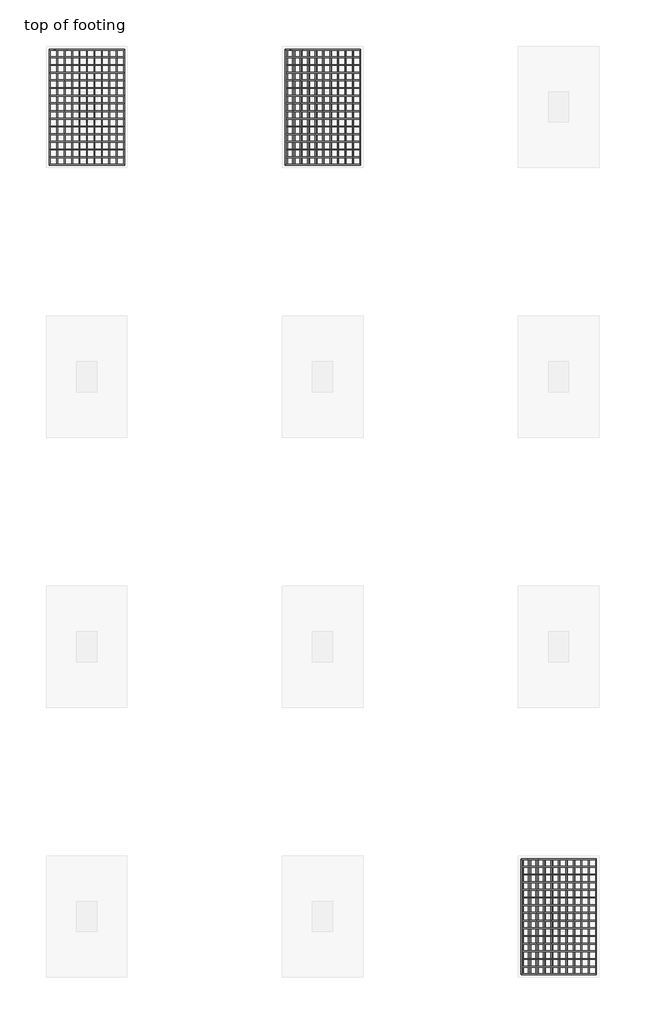
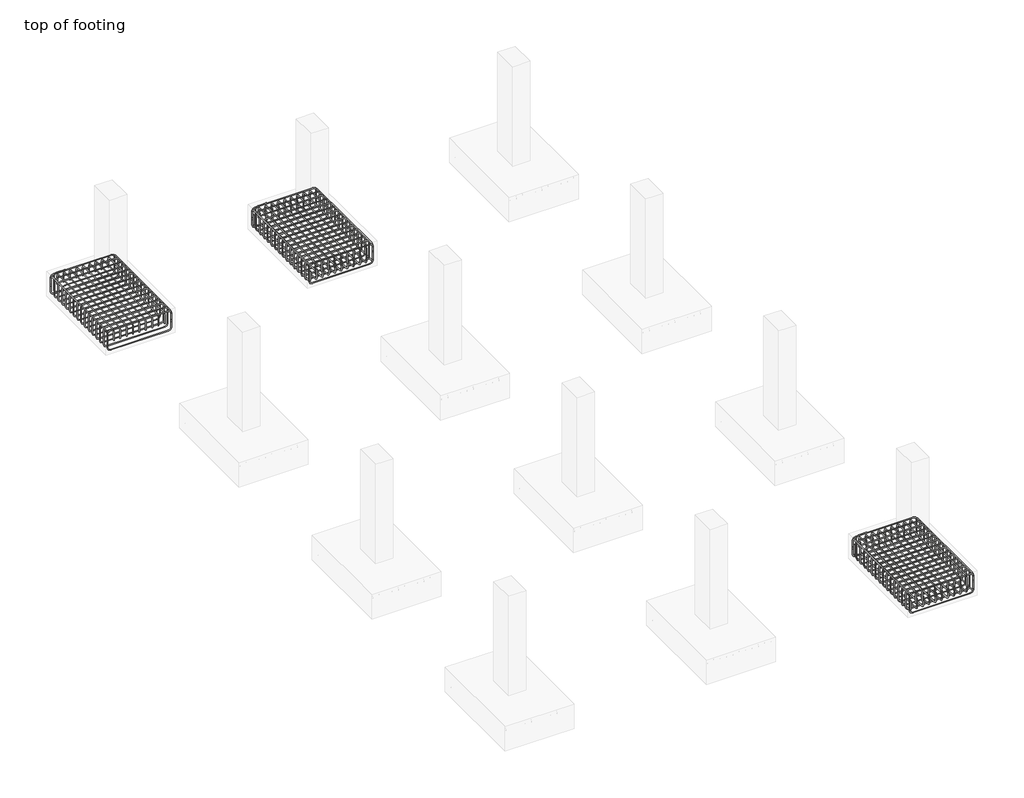
# One storey, part 7 of 8: 14 reinforcing bars.
"""IFC4 building model written with IfcOpenShell, lengths in millimetres."""

from ifc_helpers import new_model, si_unit, point, frame, origin, place, context, project, spatial, polyline, circle_curve, trimmed, segment, composite_curve, source, transform, mapped, element, save
from ifc_brep_helpers import swept_disk

model = new_model("IFC4")

# Units and contexts
model_context = context("Model", 3, world=origin())
ifc_project = project(units=[si_unit("LENGTHUNIT", "METRE", prefix="MILLI")], contexts=[model_context])

# Site, building, storey
site = spatial("IfcSite", under=ifc_project)
building = spatial("IfcBuilding", under=site)
storey = spatial("IfcBuildingStorey", under=building, Name="top of footing", Elevation=-1828.8)

# Reinforcing bars
placement = place(None, origin())
reinforcing_bar_shape = source(origin(), model_context, "Body", "SolidModel", [
    swept_disk(composite_curve([segment(polyline([(3314.5699811, 4682.8075251, -2014.4920065), (3314.5699811, 4682.8075251, -2161.7920065)]), True, "CONTINUOUS"), segment(trimmed(circle_curve(frame((3314.5699811, 4729.1575251, -2161.7920065), z_axis=(1.0, 0.0, 0.0), x_axis=(0.0, -46.350000000000364, 0.0)), 46.35), [point((3314.5699811, 4682.8075251, -2161.7920065))], [point((3314.5699811, 4729.1575251, -2208.1420065))], True, "CARTESIAN"), True, "CONTINUOUS"), segment(polyline([(3314.5699811, 4729.1575251, -2208.1420065), (3314.5699811, 6343.7575251, -2208.1420065)]), True, "CONTINUOUS"), segment(trimmed(circle_curve(frame((3314.5699811, 6343.7575251, -2161.7920065), z_axis=(1.0, 0.0, 0.0), x_axis=(0.0, 0.0, -46.350000000000364)), 46.35), [point((3314.5699811, 6343.7575251, -2208.1420065))], [point((3314.5699811, 6390.1075251, -2161.7920065))], True, "CARTESIAN"), True, "CONTINUOUS"), segment(polyline([(3314.5699811, 6390.1075251, -2161.7920065), (3314.5699811, 6390.1075251, -2014.4920065)]), True, "CONTINUOUS")], self_intersect=False), 6.35),
])
element("IfcReinforcingBar", 1, at=placement, inside=storey, context=model_context, shape_type="MappedRepresentation", body=[
    mapped(reinforcing_bar_shape, transform((0.0, 0.0, 0.0), x_axis=(1.0, 0.0, 0.0), y_axis=(0.0, 1.0, 0.0), z_axis=(0.0, 0.0, 1.0))),
    mapped(reinforcing_bar_shape, transform((-108.3645139, 0.0, 0.0), x_axis=(1.0, 0.0, 0.0), y_axis=(0.0, 1.0, 0.0), z_axis=(0.0, 0.0, 1.0))),
    mapped(reinforcing_bar_shape, transform((-216.7290279, 0.0, 0.0), x_axis=(1.0, 0.0, 0.0), y_axis=(0.0, 1.0, 0.0), z_axis=(0.0, 0.0, 1.0))),
    mapped(reinforcing_bar_shape, transform((-325.0935418, 0.0, 0.0), x_axis=(1.0, 0.0, 0.0), y_axis=(0.0, 1.0, 0.0), z_axis=(0.0, 0.0, 1.0))),
    mapped(reinforcing_bar_shape, transform((-433.4580557, 0.0, 0.0), x_axis=(1.0, 0.0, 0.0), y_axis=(0.0, 1.0, 0.0), z_axis=(0.0, 0.0, 1.0))),
    mapped(reinforcing_bar_shape, transform((-541.8225696, 0.0, 0.0), x_axis=(1.0, 0.0, 0.0), y_axis=(0.0, 1.0, 0.0), z_axis=(0.0, 0.0, 1.0))),
    mapped(reinforcing_bar_shape, transform((-650.1870836, 0.0, 0.0), x_axis=(1.0, 0.0, 0.0), y_axis=(0.0, 1.0, 0.0), z_axis=(0.0, 0.0, 1.0))),
    mapped(reinforcing_bar_shape, transform((-758.5515975, 0.0, 0.0), x_axis=(1.0, 0.0, 0.0), y_axis=(0.0, 1.0, 0.0), z_axis=(0.0, 0.0, 1.0))),
    mapped(reinforcing_bar_shape, transform((-866.9161114, 0.0, 0.0), x_axis=(1.0, 0.0, 0.0), y_axis=(0.0, 1.0, 0.0), z_axis=(0.0, 0.0, 1.0))),
    mapped(reinforcing_bar_shape, transform((-975.2806253, 0.0, 0.0), x_axis=(1.0, 0.0, 0.0), y_axis=(0.0, 1.0, 0.0), z_axis=(0.0, 0.0, 1.0))),
    mapped(reinforcing_bar_shape, transform((-1083.6451393, 0.0, 0.0), x_axis=(1.0, 0.0, 0.0), y_axis=(0.0, 1.0, 0.0), z_axis=(0.0, 0.0, 1.0))),
])
reinforcing_bar_2_shape = source(origin(), model_context, "Body", "SolidModel", [
    swept_disk(composite_curve([segment(polyline([(2207.2699811, 4682.8075251, -2085.8010212), (2207.2699811, 4682.8075251, -1938.5010212)]), True, "CONTINUOUS"), segment(trimmed(circle_curve(frame((2207.2699811, 4729.1575251, -1938.5010212), z_axis=(-1.0, 0.0, 0.0), x_axis=(0.0, -46.350000000000364, 0.0)), 46.35), [point((2207.2699811, 4682.8075251, -1938.5010212))], [point((2207.2699811, 4729.1575251, -1892.1510212))], True, "CARTESIAN"), True, "CONTINUOUS"), segment(polyline([(2207.2699811, 4729.1575251, -1892.1510212), (2207.2699811, 6343.7575251, -1892.1510212)]), True, "CONTINUOUS"), segment(trimmed(circle_curve(frame((2207.2699811, 6343.7575251, -1938.5010212), z_axis=(-1.0, 0.0, 0.0), x_axis=(0.0, 0.0, 46.34999999999991)), 46.35), [point((2207.2699811, 6343.7575251, -1892.1510212))], [point((2207.2699811, 6390.1075251, -1938.5010212))], True, "CARTESIAN"), True, "CONTINUOUS"), segment(polyline([(2207.2699811, 6390.1075251, -1938.5010212), (2207.2699811, 6390.1075251, -2085.8010212)]), True, "CONTINUOUS")], self_intersect=False), 6.35),
])
element("IfcReinforcingBar", 2, at=placement, inside=storey, context=model_context, shape_type="MappedRepresentation", body=[
    mapped(reinforcing_bar_2_shape, transform((0.0, 0.0, 0.0), x_axis=(1.0, 0.0, 0.0), y_axis=(0.0, 1.0, 0.0), z_axis=(0.0, 0.0, 1.0))),
    mapped(reinforcing_bar_2_shape, transform((110.73, 0.0, 0.0), x_axis=(1.0, 0.0, 0.0), y_axis=(0.0, 1.0, 0.0), z_axis=(0.0, 0.0, 1.0))),
    mapped(reinforcing_bar_2_shape, transform((221.46, 0.0, 0.0), x_axis=(1.0, 0.0, 0.0), y_axis=(0.0, 1.0, 0.0), z_axis=(0.0, 0.0, 1.0))),
    mapped(reinforcing_bar_2_shape, transform((332.19, 0.0, 0.0), x_axis=(1.0, 0.0, 0.0), y_axis=(0.0, 1.0, 0.0), z_axis=(0.0, 0.0, 1.0))),
    mapped(reinforcing_bar_2_shape, transform((442.92, 0.0, 0.0), x_axis=(1.0, 0.0, 0.0), y_axis=(0.0, 1.0, 0.0), z_axis=(0.0, 0.0, 1.0))),
    mapped(reinforcing_bar_2_shape, transform((553.65, 0.0, 0.0), x_axis=(1.0, 0.0, 0.0), y_axis=(0.0, 1.0, 0.0), z_axis=(0.0, 0.0, 1.0))),
    mapped(reinforcing_bar_2_shape, transform((664.38, 0.0, 0.0), x_axis=(1.0, 0.0, 0.0), y_axis=(0.0, 1.0, 0.0), z_axis=(0.0, 0.0, 1.0))),
    mapped(reinforcing_bar_2_shape, transform((775.11, 0.0, 0.0), x_axis=(1.0, 0.0, 0.0), y_axis=(0.0, 1.0, 0.0), z_axis=(0.0, 0.0, 1.0))),
    mapped(reinforcing_bar_2_shape, transform((885.84, 0.0, 0.0), x_axis=(1.0, 0.0, 0.0), y_axis=(0.0, 1.0, 0.0), z_axis=(0.0, 0.0, 1.0))),
    mapped(reinforcing_bar_2_shape, transform((996.57, 0.0, 0.0), x_axis=(1.0, 0.0, 0.0), y_axis=(0.0, 1.0, 0.0), z_axis=(0.0, 0.0, 1.0))),
    mapped(reinforcing_bar_2_shape, transform((1107.3, 0.0, 0.0), x_axis=(1.0, 0.0, 0.0), y_axis=(0.0, 1.0, 0.0), z_axis=(0.0, 0.0, 1.0))),
])
element("IfcReinforcingBar", 3, at=placement, inside=storey, context=model_context, shape_type="SolidModel", body=[
    swept_disk(composite_curve([segment(polyline([(2456.9690895, 6390.1075251, -2232.45), (2309.6690895, 6390.1075251, -2232.45)]), True, "CONTINUOUS"), segment(trimmed(circle_curve(frame((2309.6690895, 6390.1075251, -2186.1), z_axis=(0.0, 1.0, 0.0), x_axis=(0.0, 0.0, -46.34999999999991)), 46.35), [point((2309.6690895, 6390.1075251, -2232.45))], [point((2263.3190895, 6390.1075251, -2186.1))], True, "CARTESIAN"), True, "CONTINUOUS"), segment(polyline([(2263.3190895, 6390.1075251, -2186.1), (2263.3190895, 6390.1075251, -1921.5)]), True, "CONTINUOUS"), segment(trimmed(circle_curve(frame((2309.6690895, 6390.1075251, -1921.5), z_axis=(0.0, 1.0, 0.0), x_axis=(-46.350000000000364, 0.0, 0.0)), 46.35), [point((2263.3190895, 6390.1075251, -1921.5))], [point((2309.6690895, 6390.1075251, -1875.15))], True, "CARTESIAN"), True, "CONTINUOUS"), segment(polyline([(2309.6690895, 6390.1075251, -1875.15), (2456.9690895, 6390.1075251, -1875.15)]), True, "CONTINUOUS")], self_intersect=False), 6.35),
])
reinforcing_bar_3_shape = source(origin(), model_context, "Body", "SolidModel", [
    swept_disk(composite_curve([segment(polyline([(3314.5699811, 6390.1075251, -2044.8290141), (3314.5699811, 6390.1075251, -2192.1290141)]), True, "CONTINUOUS"), segment(trimmed(circle_curve(frame((3268.2199811, 6390.1075251, -2192.1290141), z_axis=(0.0, 1.0, 0.0), x_axis=(46.34999999999991, 0.0, 0.0)), 46.35), [point((3314.5699811, 6390.1075251, -2192.1290141))], [point((3268.2199811, 6390.1075251, -2238.4790141))], True, "CARTESIAN"), True, "CONTINUOUS"), segment(polyline([(3268.2199811, 6390.1075251, -2238.4790141), (2253.6199811, 6390.1075251, -2238.4790141)]), True, "CONTINUOUS"), segment(trimmed(circle_curve(frame((2253.6199811, 6390.1075251, -2192.1290141), z_axis=(0.0, 1.0, 0.0), x_axis=(0.0, 0.0, -46.34999999999991)), 46.35), [point((2253.6199811, 6390.1075251, -2238.4790141))], [point((2207.2699811, 6390.1075251, -2192.1290141))], True, "CARTESIAN"), True, "CONTINUOUS"), segment(polyline([(2207.2699811, 6390.1075251, -2192.1290141), (2207.2699811, 6390.1075251, -2044.8290141)]), True, "CONTINUOUS")], self_intersect=False), 6.35),
])
element("IfcReinforcingBar", 4, at=placement, inside=storey, context=model_context, shape_type="MappedRepresentation", body=[
    mapped(reinforcing_bar_3_shape, transform((0.0, 0.0, 0.0), x_axis=(1.0, 0.0, 0.0), y_axis=(0.0, 1.0, 0.0), z_axis=(0.0, 0.0, 1.0))),
    mapped(reinforcing_bar_3_shape, transform((0.0, -113.82, 0.0), x_axis=(1.0, 0.0, 0.0), y_axis=(0.0, 1.0, 0.0), z_axis=(0.0, 0.0, 1.0))),
    mapped(reinforcing_bar_3_shape, transform((0.0, -227.64, 0.0), x_axis=(1.0, 0.0, 0.0), y_axis=(0.0, 1.0, 0.0), z_axis=(0.0, 0.0, 1.0))),
    mapped(reinforcing_bar_3_shape, transform((0.0, -341.46, 0.0), x_axis=(1.0, 0.0, 0.0), y_axis=(0.0, 1.0, 0.0), z_axis=(0.0, 0.0, 1.0))),
    mapped(reinforcing_bar_3_shape, transform((0.0, -455.28, 0.0), x_axis=(1.0, 0.0, 0.0), y_axis=(0.0, 1.0, 0.0), z_axis=(0.0, 0.0, 1.0))),
    mapped(reinforcing_bar_3_shape, transform((0.0, -569.1, 0.0), x_axis=(1.0, 0.0, 0.0), y_axis=(0.0, 1.0, 0.0), z_axis=(0.0, 0.0, 1.0))),
    mapped(reinforcing_bar_3_shape, transform((0.0, -682.92, 0.0), x_axis=(1.0, 0.0, 0.0), y_axis=(0.0, 1.0, 0.0), z_axis=(0.0, 0.0, 1.0))),
    mapped(reinforcing_bar_3_shape, transform((0.0, -796.74, 0.0), x_axis=(1.0, 0.0, 0.0), y_axis=(0.0, 1.0, 0.0), z_axis=(0.0, 0.0, 1.0))),
    mapped(reinforcing_bar_3_shape, transform((0.0, -910.56, 0.0), x_axis=(1.0, 0.0, 0.0), y_axis=(0.0, 1.0, 0.0), z_axis=(0.0, 0.0, 1.0))),
    mapped(reinforcing_bar_3_shape, transform((0.0, -1024.38, 0.0), x_axis=(1.0, 0.0, 0.0), y_axis=(0.0, 1.0, 0.0), z_axis=(0.0, 0.0, 1.0))),
    mapped(reinforcing_bar_3_shape, transform((0.0, -1138.2, 0.0), x_axis=(1.0, 0.0, 0.0), y_axis=(0.0, 1.0, 0.0), z_axis=(0.0, 0.0, 1.0))),
    mapped(reinforcing_bar_3_shape, transform((0.0, -1252.02, 0.0), x_axis=(1.0, 0.0, 0.0), y_axis=(0.0, 1.0, 0.0), z_axis=(0.0, 0.0, 1.0))),
    mapped(reinforcing_bar_3_shape, transform((0.0, -1365.84, 0.0), x_axis=(1.0, 0.0, 0.0), y_axis=(0.0, 1.0, 0.0), z_axis=(0.0, 0.0, 1.0))),
    mapped(reinforcing_bar_3_shape, transform((0.0, -1479.66, 0.0), x_axis=(1.0, 0.0, 0.0), y_axis=(0.0, 1.0, 0.0), z_axis=(0.0, 0.0, 1.0))),
    mapped(reinforcing_bar_3_shape, transform((0.0, -1593.48, 0.0), x_axis=(1.0, 0.0, 0.0), y_axis=(0.0, 1.0, 0.0), z_axis=(0.0, 0.0, 1.0))),
    mapped(reinforcing_bar_3_shape, transform((0.0, -1707.3, 0.0), x_axis=(1.0, 0.0, 0.0), y_axis=(0.0, 1.0, 0.0), z_axis=(0.0, 0.0, 1.0))),
])
reinforcing_bar_4_shape = source(origin(), model_context, "Body", "SolidModel", [
    swept_disk(composite_curve([segment(polyline([(2207.2699811, 6390.1075251, -2075.0801535), (2207.2699811, 6390.1075251, -1927.7801535)]), True, "CONTINUOUS"), segment(trimmed(circle_curve(frame((2253.6199811, 6390.1075251, -1927.7801535), z_axis=(0.0, 1.0, 0.0), x_axis=(-46.34999999999991, 0.0, 0.0)), 46.35), [point((2207.2699811, 6390.1075251, -1927.7801535))], [point((2253.6199811, 6390.1075251, -1881.4301535))], True, "CARTESIAN"), True, "CONTINUOUS"), segment(polyline([(2253.6199811, 6390.1075251, -1881.4301535), (3268.2199811, 6390.1075251, -1881.4301535)]), True, "CONTINUOUS"), segment(trimmed(circle_curve(frame((3268.2199811, 6390.1075251, -1927.7801535), z_axis=(0.0, 1.0, 0.0), x_axis=(0.0, 0.0, 46.350000000000136)), 46.35), [point((3268.2199811, 6390.1075251, -1881.4301535))], [point((3314.5699811, 6390.1075251, -1927.7801535))], True, "CARTESIAN"), True, "CONTINUOUS"), segment(polyline([(3314.5699811, 6390.1075251, -1927.7801535), (3314.5699811, 6390.1075251, -2075.0801535)]), True, "CONTINUOUS")], self_intersect=False), 6.35),
])
element("IfcReinforcingBar", 5, at=placement, inside=storey, context=model_context, shape_type="MappedRepresentation", body=[
    mapped(reinforcing_bar_4_shape, transform((0.0, 0.0, 0.0), x_axis=(1.0, 0.0, 0.0), y_axis=(0.0, 1.0, 0.0), z_axis=(0.0, 0.0, 1.0))),
    mapped(reinforcing_bar_4_shape, transform((0.0, -113.82, 0.0), x_axis=(1.0, 0.0, 0.0), y_axis=(0.0, 1.0, 0.0), z_axis=(0.0, 0.0, 1.0))),
    mapped(reinforcing_bar_4_shape, transform((0.0, -227.64, 0.0), x_axis=(1.0, 0.0, 0.0), y_axis=(0.0, 1.0, 0.0), z_axis=(0.0, 0.0, 1.0))),
    mapped(reinforcing_bar_4_shape, transform((0.0, -341.46, 0.0), x_axis=(1.0, 0.0, 0.0), y_axis=(0.0, 1.0, 0.0), z_axis=(0.0, 0.0, 1.0))),
    mapped(reinforcing_bar_4_shape, transform((0.0, -455.28, 0.0), x_axis=(1.0, 0.0, 0.0), y_axis=(0.0, 1.0, 0.0), z_axis=(0.0, 0.0, 1.0))),
    mapped(reinforcing_bar_4_shape, transform((0.0, -569.1, 0.0), x_axis=(1.0, 0.0, 0.0), y_axis=(0.0, 1.0, 0.0), z_axis=(0.0, 0.0, 1.0))),
    mapped(reinforcing_bar_4_shape, transform((0.0, -682.92, 0.0), x_axis=(1.0, 0.0, 0.0), y_axis=(0.0, 1.0, 0.0), z_axis=(0.0, 0.0, 1.0))),
    mapped(reinforcing_bar_4_shape, transform((0.0, -796.74, 0.0), x_axis=(1.0, 0.0, 0.0), y_axis=(0.0, 1.0, 0.0), z_axis=(0.0, 0.0, 1.0))),
    mapped(reinforcing_bar_4_shape, transform((0.0, -910.56, 0.0), x_axis=(1.0, 0.0, 0.0), y_axis=(0.0, 1.0, 0.0), z_axis=(0.0, 0.0, 1.0))),
    mapped(reinforcing_bar_4_shape, transform((0.0, -1024.38, 0.0), x_axis=(1.0, 0.0, 0.0), y_axis=(0.0, 1.0, 0.0), z_axis=(0.0, 0.0, 1.0))),
    mapped(reinforcing_bar_4_shape, transform((0.0, -1138.2, 0.0), x_axis=(1.0, 0.0, 0.0), y_axis=(0.0, 1.0, 0.0), z_axis=(0.0, 0.0, 1.0))),
    mapped(reinforcing_bar_4_shape, transform((0.0, -1252.02, 0.0), x_axis=(1.0, 0.0, 0.0), y_axis=(0.0, 1.0, 0.0), z_axis=(0.0, 0.0, 1.0))),
    mapped(reinforcing_bar_4_shape, transform((0.0, -1365.84, 0.0), x_axis=(1.0, 0.0, 0.0), y_axis=(0.0, 1.0, 0.0), z_axis=(0.0, 0.0, 1.0))),
    mapped(reinforcing_bar_4_shape, transform((0.0, -1479.66, 0.0), x_axis=(1.0, 0.0, 0.0), y_axis=(0.0, 1.0, 0.0), z_axis=(0.0, 0.0, 1.0))),
    mapped(reinforcing_bar_4_shape, transform((0.0, -1593.48, 0.0), x_axis=(1.0, 0.0, 0.0), y_axis=(0.0, 1.0, 0.0), z_axis=(0.0, 0.0, 1.0))),
    mapped(reinforcing_bar_4_shape, transform((0.0, -1707.3, 0.0), x_axis=(1.0, 0.0, 0.0), y_axis=(0.0, 1.0, 0.0), z_axis=(0.0, 0.0, 1.0))),
])
reinforcing_bar_5_shape = source(origin(), model_context, "Body", "SolidModel", [
    swept_disk(composite_curve([segment(polyline([(-4792.7300189, 16682.8075251, -2085.8010212), (-4792.7300189, 16682.8075251, -1938.5010212)]), True, "CONTINUOUS"), segment(trimmed(circle_curve(frame((-4792.7300189, 16729.1575251, -1938.5010212), z_axis=(-1.0, 0.0, 0.0), x_axis=(0.0, -46.349999999998545, 0.0)), 46.35), [point((-4792.7300189, 16682.8075251, -1938.5010212))], [point((-4792.7300189, 16729.1575251, -1892.1510212))], True, "CARTESIAN"), True, "CONTINUOUS"), segment(polyline([(-4792.7300189, 16729.1575251, -1892.1510212), (-4792.7300189, 18343.7575251, -1892.1510212)]), True, "CONTINUOUS"), segment(trimmed(circle_curve(frame((-4792.7300189, 18343.7575251, -1938.5010212), z_axis=(-1.0, 0.0, 0.0), x_axis=(0.0, 0.0, 46.34999999999991)), 46.35), [point((-4792.7300189, 18343.7575251, -1892.1510212))], [point((-4792.7300189, 18390.1075251, -1938.5010212))], True, "CARTESIAN"), True, "CONTINUOUS"), segment(polyline([(-4792.7300189, 18390.1075251, -1938.5010212), (-4792.7300189, 18390.1075251, -2085.8010212)]), True, "CONTINUOUS")], self_intersect=False), 6.35),
])
element("IfcReinforcingBar", 6, at=placement, inside=storey, context=model_context, shape_type="MappedRepresentation", body=[
    mapped(reinforcing_bar_5_shape, transform((0.0, 0.0, 0.0), x_axis=(1.0, 0.0, 0.0), y_axis=(0.0, 1.0, 0.0), z_axis=(0.0, 0.0, 1.0))),
    mapped(reinforcing_bar_5_shape, transform((110.73, 0.0, 0.0), x_axis=(1.0, 0.0, 0.0), y_axis=(0.0, 1.0, 0.0), z_axis=(0.0, 0.0, 1.0))),
    mapped(reinforcing_bar_5_shape, transform((221.46, 0.0, 0.0), x_axis=(1.0, 0.0, 0.0), y_axis=(0.0, 1.0, 0.0), z_axis=(0.0, 0.0, 1.0))),
    mapped(reinforcing_bar_5_shape, transform((332.19, 0.0, 0.0), x_axis=(1.0, 0.0, 0.0), y_axis=(0.0, 1.0, 0.0), z_axis=(0.0, 0.0, 1.0))),
    mapped(reinforcing_bar_5_shape, transform((442.92, 0.0, 0.0), x_axis=(1.0, 0.0, 0.0), y_axis=(0.0, 1.0, 0.0), z_axis=(0.0, 0.0, 1.0))),
    mapped(reinforcing_bar_5_shape, transform((553.65, 0.0, 0.0), x_axis=(1.0, 0.0, 0.0), y_axis=(0.0, 1.0, 0.0), z_axis=(0.0, 0.0, 1.0))),
    mapped(reinforcing_bar_5_shape, transform((664.38, 0.0, 0.0), x_axis=(1.0, 0.0, 0.0), y_axis=(0.0, 1.0, 0.0), z_axis=(0.0, 0.0, 1.0))),
    mapped(reinforcing_bar_5_shape, transform((775.11, 0.0, 0.0), x_axis=(1.0, 0.0, 0.0), y_axis=(0.0, 1.0, 0.0), z_axis=(0.0, 0.0, 1.0))),
    mapped(reinforcing_bar_5_shape, transform((885.84, 0.0, 0.0), x_axis=(1.0, 0.0, 0.0), y_axis=(0.0, 1.0, 0.0), z_axis=(0.0, 0.0, 1.0))),
    mapped(reinforcing_bar_5_shape, transform((996.57, 0.0, 0.0), x_axis=(1.0, 0.0, 0.0), y_axis=(0.0, 1.0, 0.0), z_axis=(0.0, 0.0, 1.0))),
    mapped(reinforcing_bar_5_shape, transform((1107.3, 0.0, 0.0), x_axis=(1.0, 0.0, 0.0), y_axis=(0.0, 1.0, 0.0), z_axis=(0.0, 0.0, 1.0))),
])
element("IfcReinforcingBar", 7, at=placement, inside=storey, context=model_context, shape_type="SolidModel", body=[
    swept_disk(composite_curve([segment(polyline([(-4543.0309105, 18390.1075251, -2232.45), (-4690.3309105, 18390.1075251, -2232.45)]), True, "CONTINUOUS"), segment(trimmed(circle_curve(frame((-4690.3309105, 18390.1075251, -2186.1), z_axis=(0.0, 1.0, 0.0), x_axis=(0.0, 0.0, -46.34999999999991)), 46.35), [point((-4690.3309105, 18390.1075251, -2232.45))], [point((-4736.6809105, 18390.1075251, -2186.1))], True, "CARTESIAN"), True, "CONTINUOUS"), segment(polyline([(-4736.6809105, 18390.1075251, -2186.1), (-4736.6809105, 18390.1075251, -1921.5)]), True, "CONTINUOUS"), segment(trimmed(circle_curve(frame((-4690.3309105, 18390.1075251, -1921.5), z_axis=(0.0, 1.0, 0.0), x_axis=(-46.350000000000364, 0.0, 0.0)), 46.35), [point((-4736.6809105, 18390.1075251, -1921.5))], [point((-4690.3309105, 18390.1075251, -1875.15))], True, "CARTESIAN"), True, "CONTINUOUS"), segment(polyline([(-4690.3309105, 18390.1075251, -1875.15), (-4543.0309105, 18390.1075251, -1875.15)]), True, "CONTINUOUS")], self_intersect=False), 6.35),
])
reinforcing_bar_6_shape = source(origin(), model_context, "Body", "SolidModel", [
    swept_disk(composite_curve([segment(polyline([(-3685.4300189, 18390.1075251, -2044.8290141), (-3685.4300189, 18390.1075251, -2192.1290141)]), True, "CONTINUOUS"), segment(trimmed(circle_curve(frame((-3731.7800189, 18390.1075251, -2192.1290141), z_axis=(0.0, 1.0, 0.0), x_axis=(46.34999999999991, 0.0, 0.0)), 46.35), [point((-3685.4300189, 18390.1075251, -2192.1290141))], [point((-3731.7800189, 18390.1075251, -2238.4790141))], True, "CARTESIAN"), True, "CONTINUOUS"), segment(polyline([(-3731.7800189, 18390.1075251, -2238.4790141), (-4746.3800189, 18390.1075251, -2238.4790141)]), True, "CONTINUOUS"), segment(trimmed(circle_curve(frame((-4746.3800189, 18390.1075251, -2192.1290141), z_axis=(0.0, 1.0, 0.0), x_axis=(0.0, 0.0, -46.34999999999991)), 46.35), [point((-4746.3800189, 18390.1075251, -2238.4790141))], [point((-4792.7300189, 18390.1075251, -2192.1290141))], True, "CARTESIAN"), True, "CONTINUOUS"), segment(polyline([(-4792.7300189, 18390.1075251, -2192.1290141), (-4792.7300189, 18390.1075251, -2044.8290141)]), True, "CONTINUOUS")], self_intersect=False), 6.35),
])
element("IfcReinforcingBar", 8, at=placement, inside=storey, context=model_context, shape_type="MappedRepresentation", body=[
    mapped(reinforcing_bar_6_shape, transform((0.0, 0.0, 0.0), x_axis=(1.0, 0.0, 0.0), y_axis=(0.0, 1.0, 0.0), z_axis=(0.0, 0.0, 1.0))),
    mapped(reinforcing_bar_6_shape, transform((0.0, -113.82, 0.0), x_axis=(1.0, 0.0, 0.0), y_axis=(0.0, 1.0, 0.0), z_axis=(0.0, 0.0, 1.0))),
    mapped(reinforcing_bar_6_shape, transform((0.0, -227.64, 0.0), x_axis=(1.0, 0.0, 0.0), y_axis=(0.0, 1.0, 0.0), z_axis=(0.0, 0.0, 1.0))),
    mapped(reinforcing_bar_6_shape, transform((0.0, -341.46, 0.0), x_axis=(1.0, 0.0, 0.0), y_axis=(0.0, 1.0, 0.0), z_axis=(0.0, 0.0, 1.0))),
    mapped(reinforcing_bar_6_shape, transform((0.0, -455.28, 0.0), x_axis=(1.0, 0.0, 0.0), y_axis=(0.0, 1.0, 0.0), z_axis=(0.0, 0.0, 1.0))),
    mapped(reinforcing_bar_6_shape, transform((0.0, -569.1, 0.0), x_axis=(1.0, 0.0, 0.0), y_axis=(0.0, 1.0, 0.0), z_axis=(0.0, 0.0, 1.0))),
    mapped(reinforcing_bar_6_shape, transform((0.0, -682.92, 0.0), x_axis=(1.0, 0.0, 0.0), y_axis=(0.0, 1.0, 0.0), z_axis=(0.0, 0.0, 1.0))),
    mapped(reinforcing_bar_6_shape, transform((0.0, -796.74, 0.0), x_axis=(1.0, 0.0, 0.0), y_axis=(0.0, 1.0, 0.0), z_axis=(0.0, 0.0, 1.0))),
    mapped(reinforcing_bar_6_shape, transform((0.0, -910.56, 0.0), x_axis=(1.0, 0.0, 0.0), y_axis=(0.0, 1.0, 0.0), z_axis=(0.0, 0.0, 1.0))),
    mapped(reinforcing_bar_6_shape, transform((0.0, -1024.38, 0.0), x_axis=(1.0, 0.0, 0.0), y_axis=(0.0, 1.0, 0.0), z_axis=(0.0, 0.0, 1.0))),
    mapped(reinforcing_bar_6_shape, transform((0.0, -1138.2, 0.0), x_axis=(1.0, 0.0, 0.0), y_axis=(0.0, 1.0, 0.0), z_axis=(0.0, 0.0, 1.0))),
    mapped(reinforcing_bar_6_shape, transform((0.0, -1252.02, 0.0), x_axis=(1.0, 0.0, 0.0), y_axis=(0.0, 1.0, 0.0), z_axis=(0.0, 0.0, 1.0))),
    mapped(reinforcing_bar_6_shape, transform((0.0, -1365.84, 0.0), x_axis=(1.0, 0.0, 0.0), y_axis=(0.0, 1.0, 0.0), z_axis=(0.0, 0.0, 1.0))),
    mapped(reinforcing_bar_6_shape, transform((0.0, -1479.66, 0.0), x_axis=(1.0, 0.0, 0.0), y_axis=(0.0, 1.0, 0.0), z_axis=(0.0, 0.0, 1.0))),
    mapped(reinforcing_bar_6_shape, transform((0.0, -1593.48, 0.0), x_axis=(1.0, 0.0, 0.0), y_axis=(0.0, 1.0, 0.0), z_axis=(0.0, 0.0, 1.0))),
    mapped(reinforcing_bar_6_shape, transform((0.0, -1707.3, 0.0), x_axis=(1.0, 0.0, 0.0), y_axis=(0.0, 1.0, 0.0), z_axis=(0.0, 0.0, 1.0))),
])
reinforcing_bar_7_shape = source(origin(), model_context, "Body", "SolidModel", [
    swept_disk(composite_curve([segment(polyline([(-4792.7300189, 18390.1075251, -2075.0801535), (-4792.7300189, 18390.1075251, -1927.7801535)]), True, "CONTINUOUS"), segment(trimmed(circle_curve(frame((-4746.3800189, 18390.1075251, -1927.7801535), z_axis=(0.0, 1.0, 0.0), x_axis=(-46.349999999999454, 0.0, 0.0)), 46.35), [point((-4792.7300189, 18390.1075251, -1927.7801535))], [point((-4746.3800189, 18390.1075251, -1881.4301535))], True, "CARTESIAN"), True, "CONTINUOUS"), segment(polyline([(-4746.3800189, 18390.1075251, -1881.4301535), (-3731.7800189, 18390.1075251, -1881.4301535)]), True, "CONTINUOUS"), segment(trimmed(circle_curve(frame((-3731.7800189, 18390.1075251, -1927.7801535), z_axis=(0.0, 1.0, 0.0), x_axis=(0.0, 0.0, 46.350000000000136)), 46.35), [point((-3731.7800189, 18390.1075251, -1881.4301535))], [point((-3685.4300189, 18390.1075251, -1927.7801535))], True, "CARTESIAN"), True, "CONTINUOUS"), segment(polyline([(-3685.4300189, 18390.1075251, -1927.7801535), (-3685.4300189, 18390.1075251, -2075.0801535)]), True, "CONTINUOUS")], self_intersect=False), 6.35),
])
element("IfcReinforcingBar", 9, at=placement, inside=storey, context=model_context, shape_type="MappedRepresentation", body=[
    mapped(reinforcing_bar_7_shape, transform((0.0, 0.0, 0.0), x_axis=(1.0, 0.0, 0.0), y_axis=(0.0, 1.0, 0.0), z_axis=(0.0, 0.0, 1.0))),
    mapped(reinforcing_bar_7_shape, transform((0.0, -113.82, 0.0), x_axis=(1.0, 0.0, 0.0), y_axis=(0.0, 1.0, 0.0), z_axis=(0.0, 0.0, 1.0))),
    mapped(reinforcing_bar_7_shape, transform((0.0, -227.64, 0.0), x_axis=(1.0, 0.0, 0.0), y_axis=(0.0, 1.0, 0.0), z_axis=(0.0, 0.0, 1.0))),
    mapped(reinforcing_bar_7_shape, transform((0.0, -341.46, 0.0), x_axis=(1.0, 0.0, 0.0), y_axis=(0.0, 1.0, 0.0), z_axis=(0.0, 0.0, 1.0))),
    mapped(reinforcing_bar_7_shape, transform((0.0, -455.28, 0.0), x_axis=(1.0, 0.0, 0.0), y_axis=(0.0, 1.0, 0.0), z_axis=(0.0, 0.0, 1.0))),
    mapped(reinforcing_bar_7_shape, transform((0.0, -569.1, 0.0), x_axis=(1.0, 0.0, 0.0), y_axis=(0.0, 1.0, 0.0), z_axis=(0.0, 0.0, 1.0))),
    mapped(reinforcing_bar_7_shape, transform((0.0, -682.92, 0.0), x_axis=(1.0, 0.0, 0.0), y_axis=(0.0, 1.0, 0.0), z_axis=(0.0, 0.0, 1.0))),
    mapped(reinforcing_bar_7_shape, transform((0.0, -796.74, 0.0), x_axis=(1.0, 0.0, 0.0), y_axis=(0.0, 1.0, 0.0), z_axis=(0.0, 0.0, 1.0))),
    mapped(reinforcing_bar_7_shape, transform((0.0, -910.56, 0.0), x_axis=(1.0, 0.0, 0.0), y_axis=(0.0, 1.0, 0.0), z_axis=(0.0, 0.0, 1.0))),
    mapped(reinforcing_bar_7_shape, transform((0.0, -1024.38, 0.0), x_axis=(1.0, 0.0, 0.0), y_axis=(0.0, 1.0, 0.0), z_axis=(0.0, 0.0, 1.0))),
    mapped(reinforcing_bar_7_shape, transform((0.0, -1138.2, 0.0), x_axis=(1.0, 0.0, 0.0), y_axis=(0.0, 1.0, 0.0), z_axis=(0.0, 0.0, 1.0))),
    mapped(reinforcing_bar_7_shape, transform((0.0, -1252.02, 0.0), x_axis=(1.0, 0.0, 0.0), y_axis=(0.0, 1.0, 0.0), z_axis=(0.0, 0.0, 1.0))),
    mapped(reinforcing_bar_7_shape, transform((0.0, -1365.84, 0.0), x_axis=(1.0, 0.0, 0.0), y_axis=(0.0, 1.0, 0.0), z_axis=(0.0, 0.0, 1.0))),
    mapped(reinforcing_bar_7_shape, transform((0.0, -1479.66, 0.0), x_axis=(1.0, 0.0, 0.0), y_axis=(0.0, 1.0, 0.0), z_axis=(0.0, 0.0, 1.0))),
    mapped(reinforcing_bar_7_shape, transform((0.0, -1593.48, 0.0), x_axis=(1.0, 0.0, 0.0), y_axis=(0.0, 1.0, 0.0), z_axis=(0.0, 0.0, 1.0))),
    mapped(reinforcing_bar_7_shape, transform((0.0, -1707.3, 0.0), x_axis=(1.0, 0.0, 0.0), y_axis=(0.0, 1.0, 0.0), z_axis=(0.0, 0.0, 1.0))),
])
reinforcing_bar_8_shape = source(origin(), model_context, "Body", "SolidModel", [
    swept_disk(composite_curve([segment(polyline([(-185.4300189, 16682.8075251, -2014.4920065), (-185.4300189, 16682.8075251, -2161.7920065)]), True, "CONTINUOUS"), segment(trimmed(circle_curve(frame((-185.4300189, 16729.1575251, -2161.7920065), z_axis=(1.0, 0.0, 0.0), x_axis=(0.0, -46.349999999998545, 0.0)), 46.35), [point((-185.4300189, 16682.8075251, -2161.7920065))], [point((-185.4300189, 16729.1575251, -2208.1420065))], True, "CARTESIAN"), True, "CONTINUOUS"), segment(polyline([(-185.4300189, 16729.1575251, -2208.1420065), (-185.4300189, 18343.7575251, -2208.1420065)]), True, "CONTINUOUS"), segment(trimmed(circle_curve(frame((-185.4300189, 18343.7575251, -2161.7920065), z_axis=(1.0, 0.0, 0.0), x_axis=(0.0, 0.0, -46.350000000000364)), 46.35), [point((-185.4300189, 18343.7575251, -2208.1420065))], [point((-185.4300189, 18390.1075251, -2161.7920065))], True, "CARTESIAN"), True, "CONTINUOUS"), segment(polyline([(-185.4300189, 18390.1075251, -2161.7920065), (-185.4300189, 18390.1075251, -2014.4920065)]), True, "CONTINUOUS")], self_intersect=False), 6.35),
])
element("IfcReinforcingBar", 10, at=placement, inside=storey, context=model_context, shape_type="MappedRepresentation", body=[
    mapped(reinforcing_bar_8_shape, transform((0.0, 0.0, 0.0), x_axis=(1.0, 0.0, 0.0), y_axis=(0.0, 1.0, 0.0), z_axis=(0.0, 0.0, 1.0))),
    mapped(reinforcing_bar_8_shape, transform((-108.3645139, 0.0, 0.0), x_axis=(1.0, 0.0, 0.0), y_axis=(0.0, 1.0, 0.0), z_axis=(0.0, 0.0, 1.0))),
    mapped(reinforcing_bar_8_shape, transform((-216.7290279, 0.0, 0.0), x_axis=(1.0, 0.0, 0.0), y_axis=(0.0, 1.0, 0.0), z_axis=(0.0, 0.0, 1.0))),
    mapped(reinforcing_bar_8_shape, transform((-325.0935418, 0.0, 0.0), x_axis=(1.0, 0.0, 0.0), y_axis=(0.0, 1.0, 0.0), z_axis=(0.0, 0.0, 1.0))),
    mapped(reinforcing_bar_8_shape, transform((-433.4580557, 0.0, 0.0), x_axis=(1.0, 0.0, 0.0), y_axis=(0.0, 1.0, 0.0), z_axis=(0.0, 0.0, 1.0))),
    mapped(reinforcing_bar_8_shape, transform((-541.8225696, 0.0, 0.0), x_axis=(1.0, 0.0, 0.0), y_axis=(0.0, 1.0, 0.0), z_axis=(0.0, 0.0, 1.0))),
    mapped(reinforcing_bar_8_shape, transform((-650.1870836, 0.0, 0.0), x_axis=(1.0, 0.0, 0.0), y_axis=(0.0, 1.0, 0.0), z_axis=(0.0, 0.0, 1.0))),
    mapped(reinforcing_bar_8_shape, transform((-758.5515975, 0.0, 0.0), x_axis=(1.0, 0.0, 0.0), y_axis=(0.0, 1.0, 0.0), z_axis=(0.0, 0.0, 1.0))),
    mapped(reinforcing_bar_8_shape, transform((-866.9161114, 0.0, 0.0), x_axis=(1.0, 0.0, 0.0), y_axis=(0.0, 1.0, 0.0), z_axis=(0.0, 0.0, 1.0))),
    mapped(reinforcing_bar_8_shape, transform((-975.2806253, 0.0, 0.0), x_axis=(1.0, 0.0, 0.0), y_axis=(0.0, 1.0, 0.0), z_axis=(0.0, 0.0, 1.0))),
    mapped(reinforcing_bar_8_shape, transform((-1083.6451393, 0.0, 0.0), x_axis=(1.0, 0.0, 0.0), y_axis=(0.0, 1.0, 0.0), z_axis=(0.0, 0.0, 1.0))),
])
reinforcing_bar_9_shape = source(origin(), model_context, "Body", "SolidModel", [
    swept_disk(composite_curve([segment(polyline([(-1292.7300189, 16682.8075251, -2085.8010212), (-1292.7300189, 16682.8075251, -1938.5010212)]), True, "CONTINUOUS"), segment(trimmed(circle_curve(frame((-1292.7300189, 16729.1575251, -1938.5010212), z_axis=(-1.0, 0.0, 0.0), x_axis=(0.0, -46.349999999998545, 0.0)), 46.35), [point((-1292.7300189, 16682.8075251, -1938.5010212))], [point((-1292.7300189, 16729.1575251, -1892.1510212))], True, "CARTESIAN"), True, "CONTINUOUS"), segment(polyline([(-1292.7300189, 16729.1575251, -1892.1510212), (-1292.7300189, 18343.7575251, -1892.1510212)]), True, "CONTINUOUS"), segment(trimmed(circle_curve(frame((-1292.7300189, 18343.7575251, -1938.5010212), z_axis=(-1.0, 0.0, 0.0), x_axis=(0.0, 0.0, 46.34999999999991)), 46.35), [point((-1292.7300189, 18343.7575251, -1892.1510212))], [point((-1292.7300189, 18390.1075251, -1938.5010212))], True, "CARTESIAN"), True, "CONTINUOUS"), segment(polyline([(-1292.7300189, 18390.1075251, -1938.5010212), (-1292.7300189, 18390.1075251, -2085.8010212)]), True, "CONTINUOUS")], self_intersect=False), 6.35),
])
element("IfcReinforcingBar", 11, at=placement, inside=storey, context=model_context, shape_type="MappedRepresentation", body=[
    mapped(reinforcing_bar_9_shape, transform((0.0, 0.0, 0.0), x_axis=(1.0, 0.0, 0.0), y_axis=(0.0, 1.0, 0.0), z_axis=(0.0, 0.0, 1.0))),
    mapped(reinforcing_bar_9_shape, transform((110.73, 0.0, 0.0), x_axis=(1.0, 0.0, 0.0), y_axis=(0.0, 1.0, 0.0), z_axis=(0.0, 0.0, 1.0))),
    mapped(reinforcing_bar_9_shape, transform((221.46, 0.0, 0.0), x_axis=(1.0, 0.0, 0.0), y_axis=(0.0, 1.0, 0.0), z_axis=(0.0, 0.0, 1.0))),
    mapped(reinforcing_bar_9_shape, transform((332.19, 0.0, 0.0), x_axis=(1.0, 0.0, 0.0), y_axis=(0.0, 1.0, 0.0), z_axis=(0.0, 0.0, 1.0))),
    mapped(reinforcing_bar_9_shape, transform((442.92, 0.0, 0.0), x_axis=(1.0, 0.0, 0.0), y_axis=(0.0, 1.0, 0.0), z_axis=(0.0, 0.0, 1.0))),
    mapped(reinforcing_bar_9_shape, transform((553.65, 0.0, 0.0), x_axis=(1.0, 0.0, 0.0), y_axis=(0.0, 1.0, 0.0), z_axis=(0.0, 0.0, 1.0))),
    mapped(reinforcing_bar_9_shape, transform((664.38, 0.0, 0.0), x_axis=(1.0, 0.0, 0.0), y_axis=(0.0, 1.0, 0.0), z_axis=(0.0, 0.0, 1.0))),
    mapped(reinforcing_bar_9_shape, transform((775.11, 0.0, 0.0), x_axis=(1.0, 0.0, 0.0), y_axis=(0.0, 1.0, 0.0), z_axis=(0.0, 0.0, 1.0))),
    mapped(reinforcing_bar_9_shape, transform((885.84, 0.0, 0.0), x_axis=(1.0, 0.0, 0.0), y_axis=(0.0, 1.0, 0.0), z_axis=(0.0, 0.0, 1.0))),
    mapped(reinforcing_bar_9_shape, transform((996.57, 0.0, 0.0), x_axis=(1.0, 0.0, 0.0), y_axis=(0.0, 1.0, 0.0), z_axis=(0.0, 0.0, 1.0))),
    mapped(reinforcing_bar_9_shape, transform((1107.3, 0.0, 0.0), x_axis=(1.0, 0.0, 0.0), y_axis=(0.0, 1.0, 0.0), z_axis=(0.0, 0.0, 1.0))),
])
element("IfcReinforcingBar", 12, at=placement, inside=storey, context=model_context, shape_type="SolidModel", body=[
    swept_disk(composite_curve([segment(polyline([(-1043.0309105, 18390.1075251, -2232.45), (-1190.3309105, 18390.1075251, -2232.45)]), True, "CONTINUOUS"), segment(trimmed(circle_curve(frame((-1190.3309105, 18390.1075251, -2186.1), z_axis=(0.0, 1.0, 0.0), x_axis=(0.0, 0.0, -46.34999999999991)), 46.35), [point((-1190.3309105, 18390.1075251, -2232.45))], [point((-1236.6809105, 18390.1075251, -2186.1))], True, "CARTESIAN"), True, "CONTINUOUS"), segment(polyline([(-1236.6809105, 18390.1075251, -2186.1), (-1236.6809105, 18390.1075251, -1921.5)]), True, "CONTINUOUS"), segment(trimmed(circle_curve(frame((-1190.3309105, 18390.1075251, -1921.5), z_axis=(0.0, 1.0, 0.0), x_axis=(-46.34999999999991, 0.0, 0.0)), 46.35), [point((-1236.6809105, 18390.1075251, -1921.5))], [point((-1190.3309105, 18390.1075251, -1875.15))], True, "CARTESIAN"), True, "CONTINUOUS"), segment(polyline([(-1190.3309105, 18390.1075251, -1875.15), (-1043.0309105, 18390.1075251, -1875.15)]), True, "CONTINUOUS")], self_intersect=False), 6.35),
])
reinforcing_bar_10_shape = source(origin(), model_context, "Body", "SolidModel", [
    swept_disk(composite_curve([segment(polyline([(-185.4300189, 18390.1075251, -2044.8290141), (-185.4300189, 18390.1075251, -2192.1290141)]), True, "CONTINUOUS"), segment(trimmed(circle_curve(frame((-231.7800189, 18390.1075251, -2192.1290141), z_axis=(0.0, 1.0, 0.0), x_axis=(46.349999999999994, 0.0, 0.0)), 46.35), [point((-185.4300189, 18390.1075251, -2192.1290141))], [point((-231.7800189, 18390.1075251, -2238.4790141))], True, "CARTESIAN"), True, "CONTINUOUS"), segment(polyline([(-231.7800189, 18390.1075251, -2238.4790141), (-1246.3800189, 18390.1075251, -2238.4790141)]), True, "CONTINUOUS"), segment(trimmed(circle_curve(frame((-1246.3800189, 18390.1075251, -2192.1290141), z_axis=(0.0, 1.0, 0.0), x_axis=(0.0, 0.0, -46.34999999999991)), 46.35), [point((-1246.3800189, 18390.1075251, -2238.4790141))], [point((-1292.7300189, 18390.1075251, -2192.1290141))], True, "CARTESIAN"), True, "CONTINUOUS"), segment(polyline([(-1292.7300189, 18390.1075251, -2192.1290141), (-1292.7300189, 18390.1075251, -2044.8290141)]), True, "CONTINUOUS")], self_intersect=False), 6.35),
])
element("IfcReinforcingBar", 13, at=placement, inside=storey, context=model_context, shape_type="MappedRepresentation", body=[
    mapped(reinforcing_bar_10_shape, transform((0.0, 0.0, 0.0), x_axis=(1.0, 0.0, 0.0), y_axis=(0.0, 1.0, 0.0), z_axis=(0.0, 0.0, 1.0))),
    mapped(reinforcing_bar_10_shape, transform((0.0, -113.82, 0.0), x_axis=(1.0, 0.0, 0.0), y_axis=(0.0, 1.0, 0.0), z_axis=(0.0, 0.0, 1.0))),
    mapped(reinforcing_bar_10_shape, transform((0.0, -227.64, 0.0), x_axis=(1.0, 0.0, 0.0), y_axis=(0.0, 1.0, 0.0), z_axis=(0.0, 0.0, 1.0))),
    mapped(reinforcing_bar_10_shape, transform((0.0, -341.46, 0.0), x_axis=(1.0, 0.0, 0.0), y_axis=(0.0, 1.0, 0.0), z_axis=(0.0, 0.0, 1.0))),
    mapped(reinforcing_bar_10_shape, transform((0.0, -455.28, 0.0), x_axis=(1.0, 0.0, 0.0), y_axis=(0.0, 1.0, 0.0), z_axis=(0.0, 0.0, 1.0))),
    mapped(reinforcing_bar_10_shape, transform((0.0, -569.1, 0.0), x_axis=(1.0, 0.0, 0.0), y_axis=(0.0, 1.0, 0.0), z_axis=(0.0, 0.0, 1.0))),
    mapped(reinforcing_bar_10_shape, transform((0.0, -682.92, 0.0), x_axis=(1.0, 0.0, 0.0), y_axis=(0.0, 1.0, 0.0), z_axis=(0.0, 0.0, 1.0))),
    mapped(reinforcing_bar_10_shape, transform((0.0, -796.74, 0.0), x_axis=(1.0, 0.0, 0.0), y_axis=(0.0, 1.0, 0.0), z_axis=(0.0, 0.0, 1.0))),
    mapped(reinforcing_bar_10_shape, transform((0.0, -910.56, 0.0), x_axis=(1.0, 0.0, 0.0), y_axis=(0.0, 1.0, 0.0), z_axis=(0.0, 0.0, 1.0))),
    mapped(reinforcing_bar_10_shape, transform((0.0, -1024.38, 0.0), x_axis=(1.0, 0.0, 0.0), y_axis=(0.0, 1.0, 0.0), z_axis=(0.0, 0.0, 1.0))),
    mapped(reinforcing_bar_10_shape, transform((0.0, -1138.2, 0.0), x_axis=(1.0, 0.0, 0.0), y_axis=(0.0, 1.0, 0.0), z_axis=(0.0, 0.0, 1.0))),
    mapped(reinforcing_bar_10_shape, transform((0.0, -1252.02, 0.0), x_axis=(1.0, 0.0, 0.0), y_axis=(0.0, 1.0, 0.0), z_axis=(0.0, 0.0, 1.0))),
    mapped(reinforcing_bar_10_shape, transform((0.0, -1365.84, 0.0), x_axis=(1.0, 0.0, 0.0), y_axis=(0.0, 1.0, 0.0), z_axis=(0.0, 0.0, 1.0))),
    mapped(reinforcing_bar_10_shape, transform((0.0, -1479.66, 0.0), x_axis=(1.0, 0.0, 0.0), y_axis=(0.0, 1.0, 0.0), z_axis=(0.0, 0.0, 1.0))),
    mapped(reinforcing_bar_10_shape, transform((0.0, -1593.48, 0.0), x_axis=(1.0, 0.0, 0.0), y_axis=(0.0, 1.0, 0.0), z_axis=(0.0, 0.0, 1.0))),
    mapped(reinforcing_bar_10_shape, transform((0.0, -1707.3, 0.0), x_axis=(1.0, 0.0, 0.0), y_axis=(0.0, 1.0, 0.0), z_axis=(0.0, 0.0, 1.0))),
])
reinforcing_bar_11_shape = source(origin(), model_context, "Body", "SolidModel", [
    swept_disk(composite_curve([segment(polyline([(-1292.7300189, 18390.1075251, -2075.0801535), (-1292.7300189, 18390.1075251, -1927.7801535)]), True, "CONTINUOUS"), segment(trimmed(circle_curve(frame((-1246.3800189, 18390.1075251, -1927.7801535), z_axis=(0.0, 1.0, 0.0), x_axis=(-46.34999999999991, 0.0, 0.0)), 46.35), [point((-1292.7300189, 18390.1075251, -1927.7801535))], [point((-1246.3800189, 18390.1075251, -1881.4301535))], True, "CARTESIAN"), True, "CONTINUOUS"), segment(polyline([(-1246.3800189, 18390.1075251, -1881.4301535), (-231.7800189, 18390.1075251, -1881.4301535)]), True, "CONTINUOUS"), segment(trimmed(circle_curve(frame((-231.7800189, 18390.1075251, -1927.7801535), z_axis=(0.0, 1.0, 0.0), x_axis=(0.0, 0.0, 46.350000000000136)), 46.35), [point((-231.7800189, 18390.1075251, -1881.4301535))], [point((-185.4300189, 18390.1075251, -1927.7801535))], True, "CARTESIAN"), True, "CONTINUOUS"), segment(polyline([(-185.4300189, 18390.1075251, -1927.7801535), (-185.4300189, 18390.1075251, -2075.0801535)]), True, "CONTINUOUS")], self_intersect=False), 6.35),
])
element("IfcReinforcingBar", 14, at=placement, inside=storey, context=model_context, shape_type="MappedRepresentation", body=[
    mapped(reinforcing_bar_11_shape, transform((0.0, 0.0, 0.0), x_axis=(1.0, 0.0, 0.0), y_axis=(0.0, 1.0, 0.0), z_axis=(0.0, 0.0, 1.0))),
    mapped(reinforcing_bar_11_shape, transform((0.0, -113.82, 0.0), x_axis=(1.0, 0.0, 0.0), y_axis=(0.0, 1.0, 0.0), z_axis=(0.0, 0.0, 1.0))),
    mapped(reinforcing_bar_11_shape, transform((0.0, -227.64, 0.0), x_axis=(1.0, 0.0, 0.0), y_axis=(0.0, 1.0, 0.0), z_axis=(0.0, 0.0, 1.0))),
    mapped(reinforcing_bar_11_shape, transform((0.0, -341.46, 0.0), x_axis=(1.0, 0.0, 0.0), y_axis=(0.0, 1.0, 0.0), z_axis=(0.0, 0.0, 1.0))),
    mapped(reinforcing_bar_11_shape, transform((0.0, -455.28, 0.0), x_axis=(1.0, 0.0, 0.0), y_axis=(0.0, 1.0, 0.0), z_axis=(0.0, 0.0, 1.0))),
    mapped(reinforcing_bar_11_shape, transform((0.0, -569.1, 0.0), x_axis=(1.0, 0.0, 0.0), y_axis=(0.0, 1.0, 0.0), z_axis=(0.0, 0.0, 1.0))),
    mapped(reinforcing_bar_11_shape, transform((0.0, -682.92, 0.0), x_axis=(1.0, 0.0, 0.0), y_axis=(0.0, 1.0, 0.0), z_axis=(0.0, 0.0, 1.0))),
    mapped(reinforcing_bar_11_shape, transform((0.0, -796.74, 0.0), x_axis=(1.0, 0.0, 0.0), y_axis=(0.0, 1.0, 0.0), z_axis=(0.0, 0.0, 1.0))),
    mapped(reinforcing_bar_11_shape, transform((0.0, -910.56, 0.0), x_axis=(1.0, 0.0, 0.0), y_axis=(0.0, 1.0, 0.0), z_axis=(0.0, 0.0, 1.0))),
    mapped(reinforcing_bar_11_shape, transform((0.0, -1024.38, 0.0), x_axis=(1.0, 0.0, 0.0), y_axis=(0.0, 1.0, 0.0), z_axis=(0.0, 0.0, 1.0))),
    mapped(reinforcing_bar_11_shape, transform((0.0, -1138.2, 0.0), x_axis=(1.0, 0.0, 0.0), y_axis=(0.0, 1.0, 0.0), z_axis=(0.0, 0.0, 1.0))),
    mapped(reinforcing_bar_11_shape, transform((0.0, -1252.02, 0.0), x_axis=(1.0, 0.0, 0.0), y_axis=(0.0, 1.0, 0.0), z_axis=(0.0, 0.0, 1.0))),
    mapped(reinforcing_bar_11_shape, transform((0.0, -1365.84, 0.0), x_axis=(1.0, 0.0, 0.0), y_axis=(0.0, 1.0, 0.0), z_axis=(0.0, 0.0, 1.0))),
    mapped(reinforcing_bar_11_shape, transform((0.0, -1479.66, 0.0), x_axis=(1.0, 0.0, 0.0), y_axis=(0.0, 1.0, 0.0), z_axis=(0.0, 0.0, 1.0))),
    mapped(reinforcing_bar_11_shape, transform((0.0, -1593.48, 0.0), x_axis=(1.0, 0.0, 0.0), y_axis=(0.0, 1.0, 0.0), z_axis=(0.0, 0.0, 1.0))),
    mapped(reinforcing_bar_11_shape, transform((0.0, -1707.3, 0.0), x_axis=(1.0, 0.0, 0.0), y_axis=(0.0, 1.0, 0.0), z_axis=(0.0, 0.0, 1.0))),
])

save(model, "model.ifc")

# Revit data of these elements
# Elements 1, 2, 3, 4, 5, 6, 7, 8, 9, 10, 11, 12, 13, 14 (IfcReinforcingBar)
#   Phase Created = New Construction
